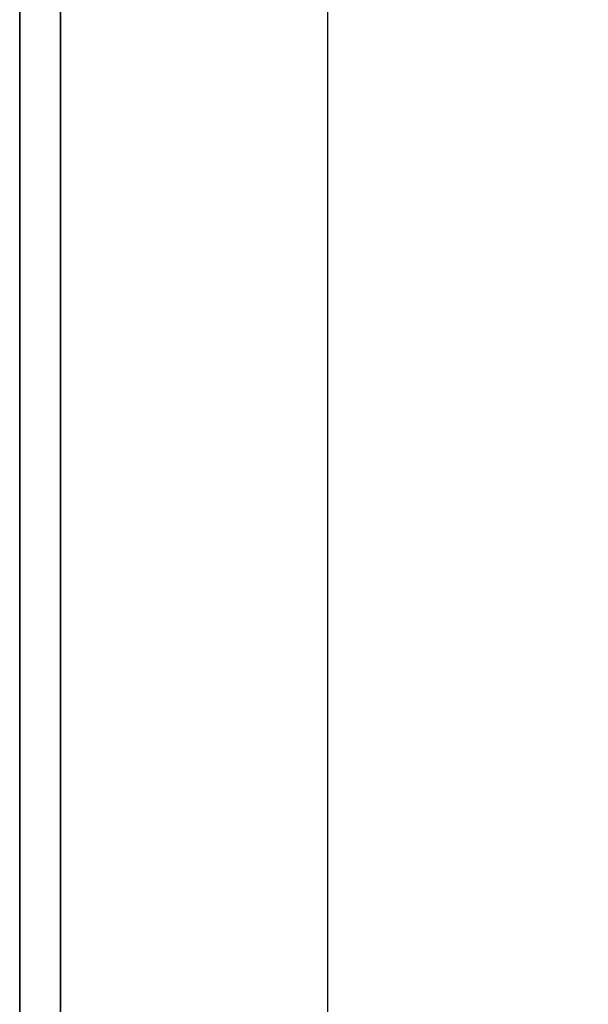
# Model space of a CAD drawing. Units: inches. Extents: x -438 to 102, y -60 to 1091.
# Tile 18 of 20: x 24 to 87, y 699 to 807. Entities that reach past the tile are written whole.
import ezdxf

# ---------------------------------------------------------------- set-up
doc = ezdxf.new("R2010")
doc.units = ezdxf.units.IN
doc.header["$MEASUREMENT"] = 0
for name, color, linetype, lineweight, true_color in [('A-ANNO-DIMS', 217, 'Continuous', 18, 0x93278f), ('A-WALL', 2, 'Continuous', 35, 0xf1eb1f), ('C-PROP', 2, 'Continuous', 35, 0xf1eb1f)]:
    doc.layers.add(name, color=color, linetype=linetype, lineweight=lineweight, true_color=true_color)
doc.styles.get("Standard").update_dxf_attribs({"font": 'arial.ttf'})
doc.dimstyles.get("Standard").update_dxf_attribs({"dimtxt": 8, "dimasz": 0.18, "dimexe": 0.18, "dimexo": 0.0625, "dimgap": 0.09, "dimtad": 0, "dimtih": 1, "dimtoh": 1, "dimdec": 4, "dimzin": 0, "dimdsep": 46, "dimlunit": 3, "dimtxsty": 'Standard', "dimcen": 0.09, "dimadec": 0, "dimazin": 0, "dimtfac": 1, "dimtdec": 4, "dimtofl": 0, "dimtmove": 0, "dimatfit": 3, "dimfxl": 1, "dimtolj": 1, "dimtzin": 0, "dimarcsym": 0})

# ---------------------------------------------------------------- blocks, each defined once
blk = doc.blocks.new('*D5')
at = {"layer": 'A-ANNO-DIMS', "color": 0, "lineweight": -2, "transparency": 16777216}
for p, q in [((28.92, 1027), (58.42, 1027)), ((58.24, 1026.82), (58.24, 519.68)), ((58.24, 4.18), (58.24, 511.32)), ((28.92, 4), (58.42, 4))]:
    blk.add_line(p, q, dxfattribs=at)
at = {"layer": 'A-ANNO-DIMS', "color": 0, "transparency": 16777216}
for points in [[(58.21, 1026.82), (58.27, 1026.82), (58.24, 1027)], [(58.21, 4.18), (58.27, 4.18), (58.24, 4)]]:
    blk.add_solid(points, dxfattribs=at)
at = {"layer": 'Defpoints', "color": 0, "transparency": 16777216}
for p in [(28.85, 1027), (28.85, 4), (58.24, 4)]:
    blk.add_point(p, dxfattribs=at)
at = {"layer": 'A-ANNO-DIMS', "color": 0, "transparency": 16777216, "insert": (58.24, 515.5), "char_height": 8, "attachment_point": 5}
blk.add_mtext('\\A1;85\'-3.0000"', dxfattribs=at)

msp = doc.modelspace()

# ---------------------------------------------------------------- linework, layer by layer
at = {"layer": 'A-WALL'}
msp.add_line((24.35351, 665.49939), (24.35351, 839.49939), dxfattribs=at)
at = {"layer": 'C-PROP'}
msp.add_line((28.85351, 3.99939), (28.85351, 1026.99939), dxfattribs=at)

# ---------------------------------------------------------------- dimensions: what is measured, and where the dimension line sits
at = {"layer": 'A-ANNO-DIMS'}
dim = msp.add_linear_dim(base=(58.24207, 3.99939), p1=(28.85351, 1026.99939), p2=(28.85351, 3.99939), angle=90, dimstyle='Standard', override={"dimclrd": 0, "dimclre": 0, "dimclrt": 0}, dxfattribs=at)
dim.commit()
dim.dimension.update_dxf_attribs({"geometry": '*D5', "text_midpoint": (58.24207, 515.49939)})

doc.saveas('drawing.dxf')
